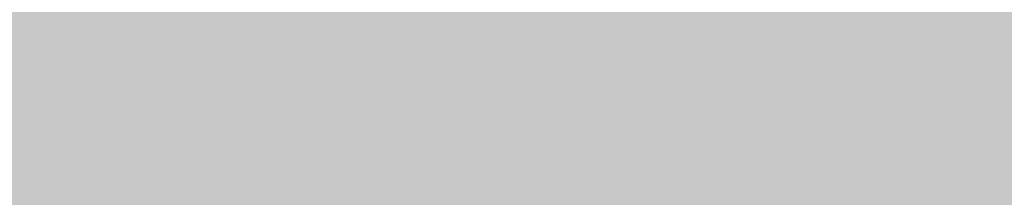
# Model space of a CAD drawing. Units: feet. Extents: x 3168 to 4724, y 827 to 1477.
# Tile 184 of 256: x 3307.378 to 3316.072, y 1096.781 to 1098.344. Entities that reach past the tile are written whole.
import ezdxf

# ---------------------------------------------------------------- set-up
doc = ezdxf.new("R2010")
doc.units = ezdxf.units.FT
doc.layers.add('A-ELEV-PATT', color=8, linetype='Continuous', lineweight=13)

msp = doc.modelspace()

# ---------------------------------------------------------------- hatches: boundary and pattern name
at = {"layer": 'A-ELEV-PATT'}
h = msp.add_hatch(color=256, dxfattribs=at)
h.dxf.hatch_style = 1
edge = h.paths.add_edge_path()
edge.add_ellipse((3552.9058, 979.2201), major_axis=(36.7449, 0), ratio=0.4848485, start_angle=0, end_angle=360)
edge = h.paths.add_edge_path()
edge.add_ellipse((3559.8916, 929.2523), major_axis=(36.7449, 0), ratio=0.4848485, start_angle=0, end_angle=360)
edge = h.paths.add_edge_path()
edge.add_line((3299.3168, 1198.6061), (3479.9167, 1198.6061))
edge.add_line((3479.9167, 1198.6061), (3479.9167, 1209.8686))
edge.add_spline(control_points=[(3479.9167, 1209.8686), (3464.3012, 1209.8686), (3448.6856, 1209.8686), (3410.9491, 1209.8686), (3388.8282, 1209.8686), (3355.6469, 1209.8686), (3344.5864, 1209.8686), (3327.9957, 1209.8686), (3322.4655, 1209.8686), (3314.1702, 1209.8686), (3311.4051, 1209.8686), (3307.2574, 1209.8686), (3305.8748, 1209.8686), (3303.801, 1209.8686), (3303.1097, 1209.8686), (3302.0728, 1209.8686), (3301.7272, 1209.8686), (3301.2087, 1209.8686), (3301.0359, 1209.8686), (3300.7767, 1209.8686), (3300.6903, 1209.8686), (3300.5606, 1209.8686), (3300.5174, 1209.8686), (3300.4526, 1209.8686), (3300.431, 1209.8686), (3300.3986, 1209.8686), (3300.3878, 1209.8686), (3300.3662, 1209.8686), (3300.3457, 1209.8686), (3300.3455, 1209.8686), (3300.3455, 1209.8686), (3300.3433, 1209.8686), (3300.3411, 1209.8686), (3300.3379, 1209.8686), (3300.3368, 1209.8686), (3300.3339, 1209.8686), (3300.3321, 1209.8686), (3300.3255, 1209.8686), (3300.3207, 1209.8686), (3300.3109, 1209.8686), (3300.306, 1209.8686), (3300.2905, 1209.8686), (3300.28, 1209.8686), (3300.2324, 1209.8688), (3300.1953, 1209.869), (3299.9511, 1209.8706), (3299.7448, 1209.8743), (3299.4368, 1209.8833), (3299.3344, 1209.8868), (3299.1811, 1209.8929), (3299.13, 1209.8951), (3298.6522, 1209.9168), (3298.2295, 1209.9457), (3297.6016, 1210.0024), (3297.3934, 1210.0235), (3297.0827, 1210.0583), (3296.9793, 1210.0705), (3296.293, 1210.1549), (3295.7181, 1210.2434), (3294.8687, 1210.3989), (3294.5877, 1210.4545), (3294.1693, 1210.5433), (3294.0304, 1210.5739), (3291.7071, 1211.1012), (3289.6536, 1211.8134), (3285.7763, 1213.564), (3283.9514, 1214.6035), (3280.5122, 1216.9801), (3278.8972, 1218.3176), (3276.3799, 1220.8295), (3275.416, 1221.9177), (3274.0393, 1223.7077), (3273.581, 1224.3495), (3273.1432, 1225.0163)], knot_values=[39.119033, 39.119033, 39.119033, 39.119033, 39.286353, 39.286353, 39.523379, 39.523379, 39.641892, 39.641892, 39.701148, 39.701148, 39.730777, 39.730777, 39.745591, 39.745591, 39.752998, 39.752998, 39.756701, 39.756701, 39.758553, 39.758553, 39.759479, 39.759479, 39.759942, 39.759942, 39.760173, 39.760173, 39.760289, 39.760289, 39.760405, 39.760405, 39.760463, 39.760463, 39.763389, 39.763389, 39.764851, 39.764851, 39.767304, 39.767304, 39.773825, 39.773825, 39.78057, 39.78057, 39.79477, 39.79477, 39.845194, 39.845194, 40.126715, 40.126715, 40.267476, 40.267476, 40.337856, 40.337856, 40.927023, 40.927023, 41.221606, 41.221606, 41.368898, 41.368898, 42.202622, 42.202622, 42.619485, 42.619485, 42.827916, 42.827916, 46.118323, 46.118323, 49.408731, 49.408731, 52.699139, 52.699139, 54.927489, 54.927489, 56.104228, 56.104228, 56.104228, 56.104228], weights=[1, 1, 1, 1, 1, 1, 1, 1, 1, 1, 1, 1, 1, 1, 1, 1, 1, 1, 1, 1, 1, 1, 1, 1, 1, 1, 1, 1, 1, 1, 1, 1, 1, 1, 1, 1, 1, 1, 1, 1, 1, 1, 1, 1, 1, 1, 1, 1, 1, 1, 1, 1, 1, 1, 1, 1, 1, 1, 1, 1, 1, 1, 1, 1, 1, 1, 1, 1, 1, 1, 1, 1, 1, 1], degree=3, periodic=0)
edge.add_line((3273.1432, 1225.0163), (3273.1432, 1099.0163))
edge.add_line((3273.1432, 1099.0163), (3299.3168, 1099.0163))
edge.add_line((3299.3168, 1099.0163), (3299.3168, 1198.6061))
edge = h.paths.add_edge_path()
edge.add_line((3304.7584, 1324.1581), (3479.9167, 1324.1581))
edge.add_line((3479.9167, 1324.1581), (3479.9167, 1335.7146))
edge.add_line((3479.9167, 1335.7146), (3269.1616, 1335.7146))
edge.add_spline(control_points=[(3269.1616, 1335.7146), (3264.0242, 1335.7146), (3258.3641, 1328.9582), (3259.2643, 1323.9003)], knot_values=[0, 0, 0, 0, 15.412191, 15.412191, 15.412191, 15.412191], degree=3, periodic=0)
edge.add_line((3259.2643, 1323.9003), (3265.5168, 1288.7691))
edge.add_line((3265.5168, 1288.7691), (3275.2651, 1261.5456))
edge.add_line((3275.2651, 1261.5456), (3304.7584, 1261.5456))
edge.add_line((3304.7584, 1261.5456), (3304.7584, 1324.1581))
h = msp.add_hatch(color=256, dxfattribs=at)
h.dxf.hatch_style = 1
h.paths.add_polyline_path([(3384.5252, 1099.0163), (3335.0292, 1099.0163), (3299.3168, 1099.0163), (3273.1432, 1099.0163), (3217.5654, 1099.0163), (3168.0693, 827.1163), (3335.0292, 827.1163)])

doc.saveas('drawing.dxf')
